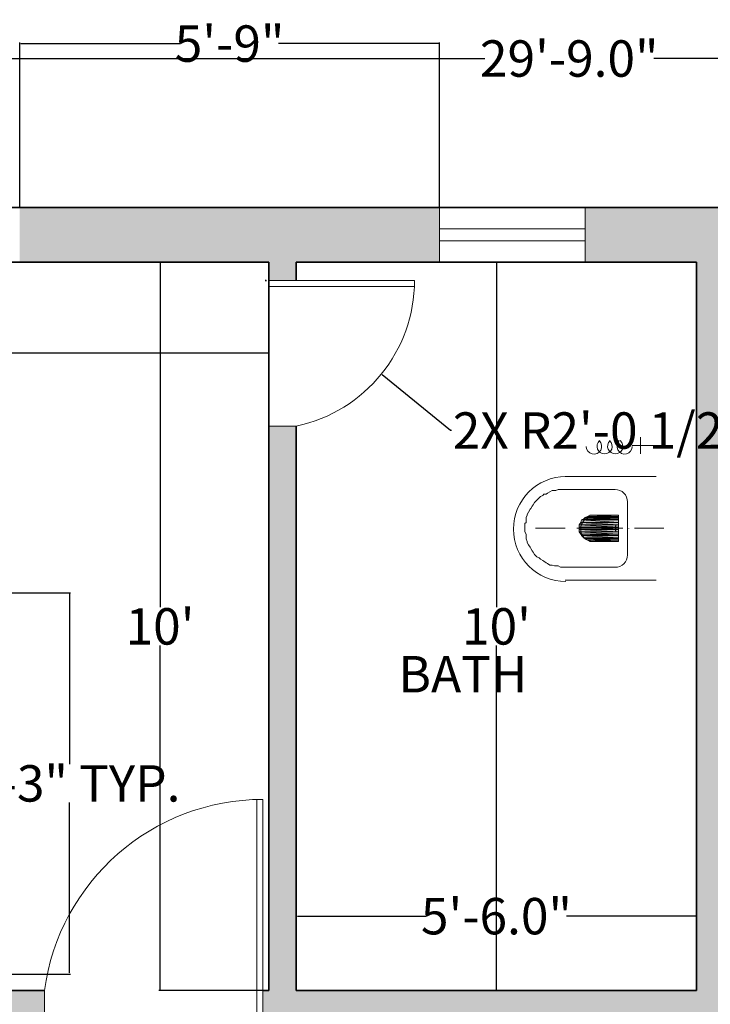
# Model space of a CAD drawing. Units: inches. Extents: x 302 to 1258, y 831 to 1373.
# Tile 10 of 13: x 934 to 1048, y 1211 to 1373. Entities that reach past the tile are written whole.
import ezdxf

# ---------------------------------------------------------------- set-up
doc = ezdxf.new("R2010")
doc.units = ezdxf.units.IN
doc.header["$MEASUREMENT"] = 0
for name, color, linetype, lineweight in [('A-ANNO-DIMS', 2, 'Continuous', 18), ('A-AREA-IDEN', 7, 'Continuous', 18), ('A-DOOR', 3, 'Continuous', 18), ('A-FLOR-FIXT', 8, 'Continuous', 18), ('A-GLAZ', 4, 'Continuous', 18), ('A-WALL', 7, 'Continuous', 35), ('A-WALL-PATT', 251, 'Continuous', 13)]:
    doc.layers.add(name, color=color, linetype=linetype, lineweight=lineweight)
doc.styles.get("Standard").update_dxf_attribs({"font": 'arial.ttf'})
doc.dimstyles.get("Standard").update_dxf_attribs({"dimtxt": 6, "dimasz": 0.18, "dimexe": 0.18, "dimexo": 0.0625, "dimgap": 0.09, "dimtad": 0, "dimtih": 1, "dimtoh": 1, "dimdec": 1, "dimzin": 0, "dimdsep": 46, "dimlunit": 3, "dimtxsty": 'Standard', "dimcen": 0.09, "dimadec": 0, "dimazin": 0, "dimtfac": 1, "dimtdec": 1, "dimtofl": 0, "dimtmove": 0, "dimatfit": 3, "dimfxl": 1, "dimtolj": 1, "dimtzin": 0, "dimarcsym": 0})

# ---------------------------------------------------------------- blocks, each defined once
blk = doc.blocks.new('*D17')
at = {"layer": 'A-ANNO-DIMS', "color": 0, "lineweight": -2, "transparency": 16777216}
for p, q in [((855.12, 1333.26), (855.12, 1318.14)), ((975.12, 1333.26), (975.12, 1318.14)), ((855.3, 1318.32), (910.22, 1318.32)), ((974.94, 1318.32), (920.02, 1318.32))]:
    blk.add_line(p, q, dxfattribs=at)
at = {"layer": 'A-ANNO-DIMS', "color": 0, "transparency": 16777216}
for points in [[(855.3, 1318.35), (855.3, 1318.29), (855.12, 1318.32)], [(974.94, 1318.35), (974.94, 1318.29), (975.12, 1318.32)]]:
    blk.add_solid(points, dxfattribs=at)
at = {"layer": 'Defpoints', "color": 0, "transparency": 16777216}
for p in [(855.12, 1333.32), (975.12, 1333.32), (975.12, 1318.32)]:
    blk.add_point(p, dxfattribs=at)
at = {"layer": 'A-ANNO-DIMS', "color": 0, "transparency": 16777216, "insert": (915.12, 1318.32), "char_height": 6, "attachment_point": 5}
blk.add_mtext("\\A1;10'", dxfattribs=at)
blk = doc.blocks.new('*D18')
at = {"layer": 'A-ANNO-DIMS', "color": 0, "lineweight": -2, "transparency": 16777216}
for p, q in [((975.06, 1333.32), (956.98, 1333.32)), ((957.16, 1333.14), (957.16, 1276.47)), ((957.16, 1213.5), (957.16, 1270.17)), ((975.06, 1213.32), (956.98, 1213.32))]:
    blk.add_line(p, q, dxfattribs=at)
at = {"layer": 'A-ANNO-DIMS', "color": 0, "transparency": 16777216}
for points in [[(957.13, 1333.14), (957.19, 1333.14), (957.16, 1333.32)], [(957.13, 1213.5), (957.19, 1213.5), (957.16, 1213.32)]]:
    blk.add_solid(points, dxfattribs=at)
at = {"layer": 'Defpoints', "color": 0, "transparency": 16777216}
for p in [(975.12, 1333.32), (957.16, 1213.32), (975.12, 1213.32)]:
    blk.add_point(p, dxfattribs=at)
at = {"layer": 'A-ANNO-DIMS', "color": 0, "transparency": 16777216, "insert": (957.16, 1273.32), "char_height": 6, "attachment_point": 5}
blk.add_mtext("\\A1;10'", dxfattribs=at)
blk = doc.blocks.new('*D19')
at = {"layer": 'A-ANNO-DIMS', "color": 0, "lineweight": -2, "transparency": 16777216}
for p, q in [((979.62, 1213.38), (979.62, 1225.77)), ((979.8, 1225.59), (1001.06, 1225.59)), ((1045.44, 1225.59), (1024.18, 1225.59)), ((1045.62, 1213.38), (1045.62, 1225.77))]:
    blk.add_line(p, q, dxfattribs=at)
at = {"layer": 'A-ANNO-DIMS', "color": 0, "transparency": 16777216}
for points in [[(979.8, 1225.62), (979.8, 1225.56), (979.62, 1225.59)], [(1045.44, 1225.62), (1045.44, 1225.56), (1045.62, 1225.59)]]:
    blk.add_solid(points, dxfattribs=at)
at = {"layer": 'Defpoints', "color": 0, "transparency": 16777216}
for p in [(979.62, 1225.59), (979.62, 1213.32), (1045.62, 1213.32)]:
    blk.add_point(p, dxfattribs=at)
at = {"layer": 'A-ANNO-DIMS', "color": 0, "transparency": 16777216, "insert": (1012.62, 1225.59), "char_height": 6, "attachment_point": 5}
blk.add_mtext('\\A1;5\'-6.0"', dxfattribs=at)
blk = doc.blocks.new('*D20')
at = {"layer": 'A-ANNO-DIMS', "color": 0, "lineweight": -2, "transparency": 16777216}
for p, q in [((1045.56, 1333.32), (1012.44, 1333.32)), ((1012.62, 1333.14), (1012.62, 1276.47)), ((1012.62, 1213.5), (1012.62, 1270.17)), ((1045.56, 1213.32), (1012.44, 1213.32))]:
    blk.add_line(p, q, dxfattribs=at)
at = {"layer": 'A-ANNO-DIMS', "color": 0, "transparency": 16777216}
for points in [[(1012.59, 1333.14), (1012.65, 1333.14), (1012.62, 1333.32)], [(1012.59, 1213.5), (1012.65, 1213.5), (1012.62, 1213.32)]]:
    blk.add_solid(points, dxfattribs=at)
at = {"layer": 'Defpoints', "color": 0, "transparency": 16777216}
for p in [(1045.62, 1333.32), (1012.62, 1213.32), (1045.62, 1213.32)]:
    blk.add_point(p, dxfattribs=at)
at = {"layer": 'A-ANNO-DIMS', "color": 0, "transparency": 16777216, "insert": (1012.62, 1273.32), "char_height": 6, "attachment_point": 5}
blk.add_mtext("\\A1;10'", dxfattribs=at)
blk = doc.blocks.new('*D33')
at = {"layer": 'A-ANNO-DIMS', "color": 0, "lineweight": -2, "transparency": 16777216}
for p, q in [((846.12, 1342.38), (846.12, 1367.04)), ((846.3, 1366.86), (1010.68, 1366.86)), ((1202.94, 1366.86), (1038.56, 1366.86)), ((1203.12, 1342.38), (1203.12, 1367.04))]:
    blk.add_line(p, q, dxfattribs=at)
at = {"layer": 'A-ANNO-DIMS', "color": 0, "transparency": 16777216}
for points in [[(846.3, 1366.89), (846.3, 1366.83), (846.12, 1366.86)], [(1202.94, 1366.89), (1202.94, 1366.83), (1203.12, 1366.86)]]:
    blk.add_solid(points, dxfattribs=at)
at = {"layer": 'Defpoints', "color": 0, "transparency": 16777216}
for p in [(1203.12, 1366.86), (846.12, 1342.32), (1203.12, 1342.32)]:
    blk.add_point(p, dxfattribs=at)
at = {"layer": 'A-ANNO-DIMS', "color": 0, "transparency": 16777216, "insert": (1024.62, 1366.86), "char_height": 6, "attachment_point": 5}
blk.add_mtext('\\A1;29\'-9.0"', dxfattribs=at)
blk = doc.blocks.new('WC-PLAN')
h = blk.add_hatch(color=256)
h.paths.add_polyline_path([(17.3, 10.16), (11.23, 10.16), (17.3, 9.71)])
h.paths.add_polyline_path([(11.23, 10.16), (17.3, 9.71), (11.08, 9.71)])
h = blk.add_hatch(color=256)
h.paths.add_polyline_path([(17.3, 10.32), (11.61, 10.32), (17.3, 10.16)])
h.paths.add_polyline_path([(11.61, 10.32), (17.3, 10.16), (11.23, 10.16)])
h = blk.add_hatch(color=256)
h.paths.add_polyline_path([(17.3, 10.54), (11.83, 10.54), (17.3, 10.32)])
h.paths.add_polyline_path([(11.83, 10.54), (17.3, 10.32), (11.61, 10.32)])
h = blk.add_hatch(color=256)
h.paths.add_polyline_path([(17.3, 10.7), (12.21, 10.7), (17.3, 10.54)])
h.paths.add_polyline_path([(12.21, 10.7), (17.3, 10.54), (11.83, 10.54)])
h = blk.add_hatch(color=256)
h.paths.add_polyline_path([(17.3, 10.92), (12.59, 10.92), (17.3, 10.7)])
h.paths.add_polyline_path([(12.59, 10.92), (17.3, 10.7), (12.21, 10.7)])
h = blk.add_hatch(color=256)
h.paths.add_polyline_path([(17.3, 9.71), (11.08, 9.71), (17.3, 9.33)])
h.paths.add_polyline_path([(11.08, 9.71), (17.3, 9.33), (10.85, 9.33)])
h = blk.add_hatch(color=256)
h.paths.add_polyline_path([(17.3, 9.33), (10.85, 9.33), (17.3, 8.95)])
h.paths.add_polyline_path([(10.85, 9.33), (17.3, 8.95), (10.85, 8.95)])
h = blk.add_hatch(color=256)
h.paths.add_polyline_path([(17.3, 8.95), (10.85, 8.95), (17.3, 8.57)])
h.paths.add_polyline_path([(10.85, 8.95), (17.3, 8.57), (10.85, 8.57)])
h = blk.add_hatch(color=256)
h.paths.add_polyline_path([(17.3, 8.57), (10.85, 8.57), (17.3, 8.19)])
h.paths.add_polyline_path([(10.85, 8.57), (17.3, 8.19), (10.85, 8.19)])
h = blk.add_hatch(color=256)
h.paths.add_polyline_path([(17.3, 8.19), (10.85, 8.19), (17.3, 7.81)])
h.paths.add_polyline_path([(10.85, 8.19), (17.3, 7.81), (11.08, 7.81)])
h = blk.add_hatch(color=256)
h.paths.add_polyline_path([(17.3, 7.81), (11.08, 7.81), (17.3, 7.59)])
h.paths.add_polyline_path([(11.08, 7.81), (17.3, 7.59), (11.23, 7.59)])
h = blk.add_hatch(color=256)
h.paths.add_polyline_path([(17.3, 7.59), (11.23, 7.59), (17.3, 7.21)])
h.paths.add_polyline_path([(11.23, 7.59), (17.3, 7.21), (11.61, 7.21)])
h = blk.add_hatch(color=256)
h.paths.add_polyline_path([(17.3, 7.21), (11.61, 7.21), (17.3, 7.05)])
h.paths.add_polyline_path([(11.61, 7.21), (17.3, 7.05), (11.83, 7.05)])
h = blk.add_hatch(color=256)
h.paths.add_polyline_path([(17.3, 7.05), (11.83, 7.05), (17.3, 6.83)])
h.paths.add_polyline_path([(11.83, 7.05), (17.3, 6.83), (12.21, 6.83)])
h = blk.add_hatch(color=256)
h.paths.add_polyline_path([(17.3, 6.83), (12.21, 6.83), (17.3, 6.6)])
h.paths.add_polyline_path([(12.21, 6.83), (17.3, 6.6), (12.59, 6.6)])
h.paths.add_polyline_path([(17.3, 6.6), (12.59, 6.6), (12.97, 6.6)])
for points in [[(20.94, 21.03), (20.94, 23.77), (20.94, 23.77)], [(25.41, 22.4), (19.57, 22.4), (19.57, 22.4)], [(23.52, 17.3), (8.5, 17.3), (8.5, 17.3)], [(9.48, 2.35), (8.72, 2.35), (8.12, 2.35), (7.74, 2.35), (7.36, 2.58), (6.98, 2.58), (6.75, 2.58), (6.37, 2.73), (5.99, 2.73), (5.61, 2.96), (5.39, 3.11), (5.01, 3.34), (4.85, 3.49), (4.48, 3.72), (4.25, 3.94), (3.87, 4.1), (3.64, 4.32), (3.49, 4.48), (3.26, 4.85), (3.11, 5.08), (2.88, 5.46), (2.73, 5.69), (2.5, 6.07), (2.28, 6.45), (2.28, 6.6), (2.12, 7.05), (2.12, 7.43), (2.12, 7.81), (1.9, 8.19), (1.9, 8.8), (1.9, 9.56), (2.12, 9.71), (2.12, 10.16), (2.12, 10.54), (2.28, 10.92), (2.28, 11.07), (2.5, 11.45), (2.73, 11.91), (2.88, 12.06), (3.11, 12.44), (3.26, 12.67), (3.49, 13.05), (3.64, 13.2), (3.87, 13.43), (4.25, 13.81), (4.48, 14.03), (4.85, 14.18), (5.01, 14.41), (5.39, 14.41), (5.61, 14.56), (5.99, 14.79), (6.37, 15.02), (6.75, 15.02), (6.98, 15.02), (7.36, 15.17), (7.74, 15.17), (8.12, 15.17), (8.72, 15.17), (9.48, 15.17)], [(16.69, 15.17), (9.48, 15.17), (9.48, 15.17)], [(18.81, 4.48), (18.81, 13.2), (18.81, 13.2)], [(17.3, 10.92), (12.97, 10.92), (12.97, 10.92)], [(17.3, 6.6), (17.3, 10.92), (17.3, 10.92)], [(8.5, 8.8), (3.64, 8.8), (3.64, 8.8)], [(18.05, 8.8), (10.47, 8.8), (10.47, 8.8)], [(16.84, 9.18), (16.92, 9.18), (16.92, 9.18)], [(16.84, 8.8), (16.84, 8.95), (16.84, 9.18)], [(16.84, 8.8), (16.92, 8.72), (16.92, 8.72)], [(16.84, 8.34), (16.84, 8.57), (16.84, 8.8)], [(16.84, 8.34), (16.92, 8.34), (16.92, 8.34)], [(19.04, 8.8), (19.04, 8.72), (19.04, 8.72)], [(24.81, 8.8), (19.95, 8.8), (19.95, 8.8)], [(17.3, 6.6), (12.97, 6.6), (12.97, 6.6)], [(16.69, 2.35), (9.48, 2.35), (9.48, 2.35)], [(23.52, 0.23), (8.5, 0.23), (8.5, 0.23)]]:
    blk.add_lwpolyline(points)
for points in [[(11.23, 10.16), (17.3, 9.71), (11.08, 9.71)], [(11.61, 10.32), (17.3, 10.16), (11.23, 10.16)], [(17.3, 10.16), (11.23, 10.16), (17.3, 9.71)], [(11.83, 10.54), (17.3, 10.32), (11.61, 10.32)], [(17.3, 10.32), (11.61, 10.32), (17.3, 10.16)], [(12.21, 10.7), (17.3, 10.54), (11.83, 10.54)], [(17.3, 10.54), (11.83, 10.54), (17.3, 10.32)], [(12.59, 10.92), (17.3, 10.7), (12.21, 10.7)], [(17.3, 10.7), (12.21, 10.7), (17.3, 10.54)], [(12.97, 10.92), (17.3, 10.92), (12.59, 10.92)], [(17.3, 10.92), (12.59, 10.92), (17.3, 10.7)], [(17.3, 10.92), (12.97, 10.92)], [(11.08, 9.71), (17.3, 9.33), (10.85, 9.33)], [(17.3, 9.33), (10.85, 9.33), (17.3, 8.95)], [(10.85, 9.33), (17.3, 8.95), (10.85, 8.95)], [(17.3, 8.95), (10.85, 8.95), (17.3, 8.57)], [(10.85, 8.95), (17.3, 8.57), (10.85, 8.57)], [(17.3, 8.57), (10.85, 8.57), (17.3, 8.19)], [(10.85, 8.57), (17.3, 8.19), (10.85, 8.19)], [(17.3, 8.19), (10.85, 8.19), (17.3, 7.81)], [(10.85, 8.19), (17.3, 7.81), (11.08, 7.81)], [(17.3, 9.71), (11.08, 9.71), (17.3, 9.33)], [(17.3, 7.81), (11.08, 7.81), (17.3, 7.59)], [(11.08, 7.81), (17.3, 7.59), (11.23, 7.59)], [(17.3, 7.59), (11.23, 7.59), (17.3, 7.21)], [(11.23, 7.59), (17.3, 7.21), (11.61, 7.21)], [(17.3, 7.21), (11.61, 7.21), (17.3, 7.05)], [(11.61, 7.21), (17.3, 7.05), (11.83, 7.05)], [(17.3, 7.05), (11.83, 7.05), (17.3, 6.83)], [(11.83, 7.05), (17.3, 6.83), (12.21, 6.83)], [(17.3, 6.83), (12.21, 6.83), (17.3, 6.6)], [(12.21, 6.83), (17.3, 6.6), (12.59, 6.6)], [(17.3, 6.6), (12.59, 6.6), (12.97, 6.6)], [(12.59, 6.6), (17.3, 6.6), (17.3, 6.6)]]:
    blk.add_lwpolyline(points, close=True)
for points, knots in [([(11.99, 22.25), (11.99, 21.72), (12.44, 21.19), (12.97, 21.03), (12.97, 21.03), (13.5, 20.88), (14.11, 21.19), (14.41, 21.64), (14.41, 21.64), (14.64, 22.17), (14.56, 22.78), (14.19, 23.16)], [0, 0, 0, 0, 0.083333, 0.083333, 0.083333, 0.083334, 0.166667, 0.166667, 0.166667, 0.166668, 1, 1, 1, 1]), ([(14.19, 23.23), (13.81, 22.86), (13.65, 22.32), (13.88, 21.79), (13.88, 21.79), (14.03, 21.34), (14.49, 21.03), (15.02, 21.03), (15.02, 21.03), (15.55, 21.03), (16.01, 21.34), (16.23, 21.79), (16.23, 21.79), (16.39, 22.32), (16.23, 22.86), (15.85, 23.23)], [0, 0, 0, 0, 0.0625, 0.0625, 0.0625, 0.062501, 0.125, 0.125, 0.125, 0.125001, 0.1875, 0.1875, 0.1875, 0.187501, 1, 1, 1, 1]), ([(15.93, 23.16), (15.55, 22.86), (15.4, 22.25), (15.63, 21.79), (15.63, 21.79), (15.78, 21.34), (16.31, 21.03), (16.76, 21.03), (16.76, 21.03), (17.3, 21.03), (17.75, 21.34), (17.98, 21.79), (17.98, 21.79), (18.13, 22.32), (17.98, 22.86), (17.6, 23.23)], [0, 0, 0, 0, 0.0625, 0.0625, 0.0625, 0.062501, 0.125, 0.125, 0.125, 0.125001, 0.1875, 0.1875, 0.1875, 0.187501, 1, 1, 1, 1]), ([(17.45, 23.23), (17.07, 22.86), (16.92, 22.17), (17.22, 21.72), (17.22, 21.72), (17.52, 21.19), (18.05, 20.88), (18.66, 21.03), (18.66, 21.03), (19.19, 21.19), (19.57, 21.72), (19.57, 22.25)], [0, 0, 0, 0, 0.083333, 0.083333, 0.083333, 0.083334, 0.166667, 0.166667, 0.166667, 0.166668, 1, 1, 1, 1]), ([(8.65, 17.3), (3.87, 17.3), (0, 13.43), (0, 8.65), (0, 8.65), (0, 3.87), (3.87, 0), (8.65, 0)], [0, 0, 0, 0, 0.125, 0.125, 0.125, 0.125001, 1, 1, 1, 1]), ([(13.12, 10.7), (11.99, 10.7), (11.08, 9.79), (11.08, 8.65), (11.08, 8.65), (11.08, 7.51), (11.99, 6.6), (13.12, 6.6)], [0, 0, 0, 0, 0.125, 0.125, 0.125, 0.125001, 1, 1, 1, 1])]:
    blk.add_open_spline(points, degree=3, knots=knots)
for points in [[(18.81, 13.12), (18.81, 14.26), (17.9, 15.17), (16.76, 15.17)], [(16.76, 2.35), (17.9, 2.35), (18.81, 3.26), (18.81, 4.4)]]:
    blk.add_open_spline(points, degree=3)
blk = doc.blocks.new('VENT-WINDOW-24IN')
for p, q in [((0, 24), (9, 24)), ((0, 0), (0, 24)), ((3.5, 0), (3.5, 24)), ((5.5, 24), (5.5, 0)), ((9, 24), (9, 0)), ((9, 0), (0, 0))]:
    blk.add_line(p, q)
blk = doc.blocks.new('DOOR-36IN-BEDROOM')
for p, q in [((35, 36), (35, 0)), ((36, 0), (36, 36)), ((36, 36), (36, 0)), ((0, 0), (0, 4.5)), ((36, 0), (0, 0)), ((37, 0), (36, 0))]:
    blk.add_line(p, q)
blk.add_arc((36, -0.32), 36.32, 90, 172.3719)
blk = doc.blocks.new('DOOR-24IN-BATH')
for p, q in [((0, 27), (0, 24)), ((0, 24), (24, 24)), ((24, 24), (0, 24)), ((0, 24), (0, 0)), ((24, 23), (0, 23)), ((0, 0), (4.5, 0))]:
    blk.add_line(p, q)
blk.add_arc((-0.52, 24), 24.52, 281.8123, 0)
blk = doc.blocks.new('*D51')
at = {"layer": 'A-ANNO-DIMS', "color": 0, "lineweight": -2, "transparency": 16777216}
for p, q in [((863.2, 1216), (863.2, 1205.58)), ((931.91, 1216), (931.91, 1205.58)), ((863.38, 1205.76), (931.73, 1205.76)), ((931.91, 1205.76), (932.09, 1205.76))]:
    blk.add_line(p, q, dxfattribs=at)
at = {"layer": 'A-ANNO-DIMS', "color": 0, "transparency": 16777216}
for points in [[(863.38, 1205.79), (863.38, 1205.73), (863.2, 1205.76)], [(931.73, 1205.79), (931.73, 1205.73), (931.91, 1205.76)]]:
    blk.add_solid(points, dxfattribs=at)
at = {"layer": 'Defpoints', "color": 0, "transparency": 16777216}
for p in [(863.2, 1216.06), (931.91, 1216.06), (931.91, 1205.76)]:
    blk.add_point(p, dxfattribs=at)
at = {"layer": 'A-ANNO-DIMS', "color": 0, "transparency": 16777216, "insert": (976.42, 1205.76), "char_height": 6, "attachment_point": 5}
blk.add_mtext('\\A1;BED SET 5\'-8 1/2" TYP.', dxfattribs=at)
blk = doc.blocks.new('*D52')
at = {"layer": 'A-ANNO-DIMS', "color": 0, "lineweight": -2, "transparency": 16777216}
for p, q in [((931.98, 1278.85), (942.4, 1278.85)), ((942.22, 1278.67), (942.22, 1250.61)), ((942.22, 1216.24), (942.22, 1244.3)), ((931.98, 1216.06), (942.4, 1216.06))]:
    blk.add_line(p, q, dxfattribs=at)
at = {"layer": 'A-ANNO-DIMS', "color": 0, "transparency": 16777216}
for points in [[(942.19, 1278.67), (942.25, 1278.67), (942.22, 1278.85)], [(942.19, 1216.24), (942.25, 1216.24), (942.22, 1216.06)]]:
    blk.add_solid(points, dxfattribs=at)
at = {"layer": 'Defpoints', "color": 0, "transparency": 16777216}
for p in [(931.91, 1278.85), (942.22, 1278.85), (931.91, 1216.06)]:
    blk.add_point(p, dxfattribs=at)
at = {"layer": 'A-ANNO-DIMS', "color": 0, "transparency": 16777216, "insert": (942.22, 1247.46), "char_height": 6, "attachment_point": 5}
blk.add_mtext('\\A1;5\'-3" TYP.', dxfattribs=at)
blk = doc.blocks.new('*D86')
at = {"layer": 'A-ANNO-DIMS', "color": 0, "lineweight": -2, "transparency": 16777216}
for p, q in [((934.03, 1342.38), (934.03, 1369.5)), ((934.21, 1369.32), (960.56, 1369.32)), ((1003.05, 1369.32), (976.69, 1369.32)), ((1003.23, 1342.38), (1003.23, 1369.5))]:
    blk.add_line(p, q, dxfattribs=at)
at = {"layer": 'A-ANNO-DIMS', "color": 0, "transparency": 16777216}
for points in [[(934.21, 1369.35), (934.21, 1369.29), (934.03, 1369.32)], [(1003.05, 1369.35), (1003.05, 1369.29), (1003.23, 1369.32)]]:
    blk.add_solid(points, dxfattribs=at)
at = {"layer": 'Defpoints', "color": 0, "transparency": 16777216}
for p in [(1003.23, 1369.32), (934.03, 1342.32), (1003.23, 1342.32)]:
    blk.add_point(p, dxfattribs=at)
at = {"layer": 'A-ANNO-DIMS', "color": 0, "transparency": 16777216, "insert": (968.63, 1369.32), "char_height": 6, "attachment_point": 5}
blk.add_mtext('\\A1;5\'-9"', dxfattribs=at)
blk = doc.blocks.new('*D97')
at = {"layer": 'A-ANNO-DIMS', "color": 0, "lineweight": -2, "transparency": 16777216}
for p, q in [((974.51, 1330.32), (974.69, 1330.32)), ((974.6, 1330.23), (974.6, 1330.41)), ((1005.05, 1305.58), (993.77, 1314.74)), ((1005.23, 1305.58), (1005.05, 1305.58))]:
    blk.add_line(p, q, dxfattribs=at)
at = {"layer": 'A-ANNO-DIMS', "color": 0, "transparency": 16777216}
blk.add_solid([(993.79, 1314.77), (993.75, 1314.72), (993.63, 1314.86)], dxfattribs=at)
at = {"layer": 'Defpoints', "color": 0, "transparency": 16777216}
for p in [(974.6, 1330.32), (993.63, 1314.86)]:
    blk.add_point(p, dxfattribs=at)
at = {"layer": 'A-ANNO-DIMS', "color": 0, "transparency": 16777216, "insert": (1029.65, 1305.58), "char_height": 6, "attachment_point": 5}
blk.add_mtext('\\A1;2X R2\'-0 1/2"', dxfattribs=at)

msp = doc.modelspace()

# ---------------------------------------------------------------- hatches: boundary and pattern name
at = {"layer": 'A-WALL-PATT'}
h = msp.add_hatch(color=256, dxfattribs=at)
h.dxf.hatch_style = 1
h.paths.add_polyline_path([(1003.23, 1342.32), (934.03, 1342.32), (934.03, 1333.32), (975.12, 1333.32), (975.12, 1330.32), (979.62, 1330.32), (979.62, 1333.32), (1003.23, 1333.32)])
h.paths.add_polyline_path([(1203.12, 1342.32), (1027.23, 1342.32), (1027.23, 1333.32), (1045.62, 1333.32), (1045.62, 1213.32), (979.62, 1213.32), (979.62, 1306.32), (975.12, 1306.32), (975.12, 1213.32), (974.12, 1213.32), (974.12, 1208.82), (975.12, 1208.82), (1051.12, 1208.82), (1051.12, 1213.32), (1050.12, 1213.32), (1050.12, 1333.32), (1194.12, 1333.32), (1194.12, 1302.71), (1203.12, 1302.71)])
h.paths.add_polyline_path([(855.12, 1333.32), (886.03, 1333.32), (886.03, 1342.32), (846.12, 1342.32), (846.12, 1300.76), (855.12, 1300.76)])
h.paths.add_polyline_path([(938.12, 1213.32), (855.12, 1213.32), (855.12, 1252.76), (846.12, 1252.76), (846.12, 1164.55), (855.12, 1164.55), (855.12, 1208.82), (933.12, 1208.82), (933.12, 1082.82), (937.62, 1082.82), (937.62, 1208.82), (938.12, 1208.82)])
h.paths.add_polyline_path([(855.12, 1116.55), (846.12, 1116.55), (846.12, 1024.44), (855.12, 1024.44)])
h.paths.add_polyline_path([(855.12, 976.44), (846.12, 976.44), (846.12, 944.2), (855.12, 944.2)])

# ---------------------------------------------------------------- linework, layer by layer
at = {"layer": 'A-WALL'}
for p, q in [((846.12, 1342.32), (1203.12, 1342.32)), ((855.12, 1333.32), (975.12, 1333.32)), ((975.12, 1333.32), (975.12, 1213.32)), ((979.62, 1333.32), (1045.62, 1333.32)), ((979.62, 1333.32), (979.62, 1330.32)), ((1045.62, 1333.32), (1045.62, 1213.32)), ((979.62, 1306.32), (979.62, 1213.32)), ((855.12, 1213.32), (938.12, 1213.32)), ((974.12, 1213.32), (975.12, 1213.32)), ((979.62, 1213.32), (1045.62, 1213.32))]:
    msp.add_line(p, q, dxfattribs=at)

# ---------------------------------------------------------------- block references
at = {"layer": 'A-DOOR'}
for name, p in [('DOOR-24IN-BATH', (975.12, 1306.32)), ('DOOR-36IN-BEDROOM', (938.12, 1208.82))]:
    msp.add_blockref(name, p, dxfattribs=at)
at = {"layer": 'A-FLOR-FIXT'}
msp.add_blockref('WC-PLAN', (1015.42, 1280.7), dxfattribs=at)
at = {"layer": 'A-GLAZ', "rotation": 269.9999999999994}
msp.add_blockref('VENT-WINDOW-24IN', (1003.23, 1342.32), dxfattribs=at)

# ---------------------------------------------------------------- texts
at = {"layer": 'A-AREA-IDEN', "insert": (996.46, 1268.44), "char_height": 6, "attachment_point": 1}
msp.add_mtext_dynamic_manual_height_columns('BATH', width=33.1895, gutter_width=30, heights=[0], dxfattribs=at)

# ---------------------------------------------------------------- dimensions: what is measured, and where the dimension line sits
at = {"layer": 'A-ANNO-DIMS'}
for base, p1, p2, override, picture, middle in [((1003.23, 1369.32), (934.03, 1342.32), (1003.23, 1342.32), {"dimdec": 1, "dimlfac": 1, "dimrnd": 0, "dimzin": 1, "dimdsep": 46, "dimlunit": 4, "dimfrac": 2}, '*D86', (968.63, 1369.32)), ((1203.12, 1366.86), (846.12, 1342.32), (1203.12, 1342.32), {"dimclrd": 0, "dimclre": 0, "dimclrt": 0}, '*D33', (1024.62, 1366.86)), ((975.12, 1318.32), (855.12, 1333.32), (975.12, 1333.32), {"dimclrd": 0, "dimclre": 0, "dimclrt": 0}, '*D17', (915.12, 1318.32)), ((979.62, 1225.59), (1045.62, 1213.32), (979.62, 1213.32), {"dimclrd": 0, "dimclre": 0, "dimclrt": 0}, '*D19', (1012.62, 1225.59))]:
    dim = msp.add_linear_dim(base=base, p1=p1, p2=p2, dimstyle='Standard', override=override, dxfattribs=at)
    dim.commit()
    dim.dimension.update_dxf_attribs({"geometry": picture, "text_midpoint": middle})
for base, p1, p2, picture, middle in [((957.16, 1213.32), (975.12, 1333.32), (975.12, 1213.32), '*D18', (957.16, 1273.32)), ((1012.62, 1213.32), (1045.62, 1333.32), (1045.62, 1213.32), '*D20', (1012.62, 1273.32))]:
    dim = msp.add_linear_dim(base=base, p1=p1, p2=p2, angle=90, dimstyle='Standard', override={"dimclrd": 0, "dimclre": 0, "dimclrt": 0}, dxfattribs=at)
    dim.commit()
    dim.dimension.update_dxf_attribs({"geometry": picture, "text_midpoint": middle})
dim = msp.add_radius_dim(center=(974.6, 1330.32), mpoint=(993.63, 1314.86), text='2X <>', dimstyle='Standard', override={"dimdec": 1, "dimlfac": 1, "dimrnd": 0, "dimzin": 1, "dimdsep": 46, "dimlunit": 4, "dimfrac": 2}, dxfattribs=at)
dim.commit()
dim.dimension.update_dxf_attribs({"geometry": '*D97', "text_midpoint": (1029.65, 1305.58), "dimtype": 164})
dim = msp.add_linear_dim(base=(942.22, 1278.85), p1=(931.91, 1216.06), p2=(931.91, 1278.85), angle=90, text='<> TYP.', dimstyle='Standard', override={"dimdec": 1, "dimlfac": 1, "dimrnd": 0, "dimzin": 1, "dimdsep": 46, "dimlunit": 4, "dimfrac": 2}, dxfattribs=at)
dim.commit()
dim.dimension.update_dxf_attribs({"geometry": '*D52', "text_midpoint": (942.22, 1247.46)})
dim = msp.add_linear_dim(base=(931.91, 1205.76), p1=(863.2, 1216.06), p2=(931.91, 1216.06), text='BED SET <> TYP.', dimstyle='Standard', override={"dimdec": 1, "dimlfac": 1, "dimrnd": 0, "dimzin": 1, "dimdsep": 46, "dimlunit": 4, "dimfrac": 2}, dxfattribs=at)
dim.commit()
dim.dimension.update_dxf_attribs({"geometry": '*D51', "text_midpoint": (976.42, 1205.76)})

doc.saveas('drawing.dxf')
